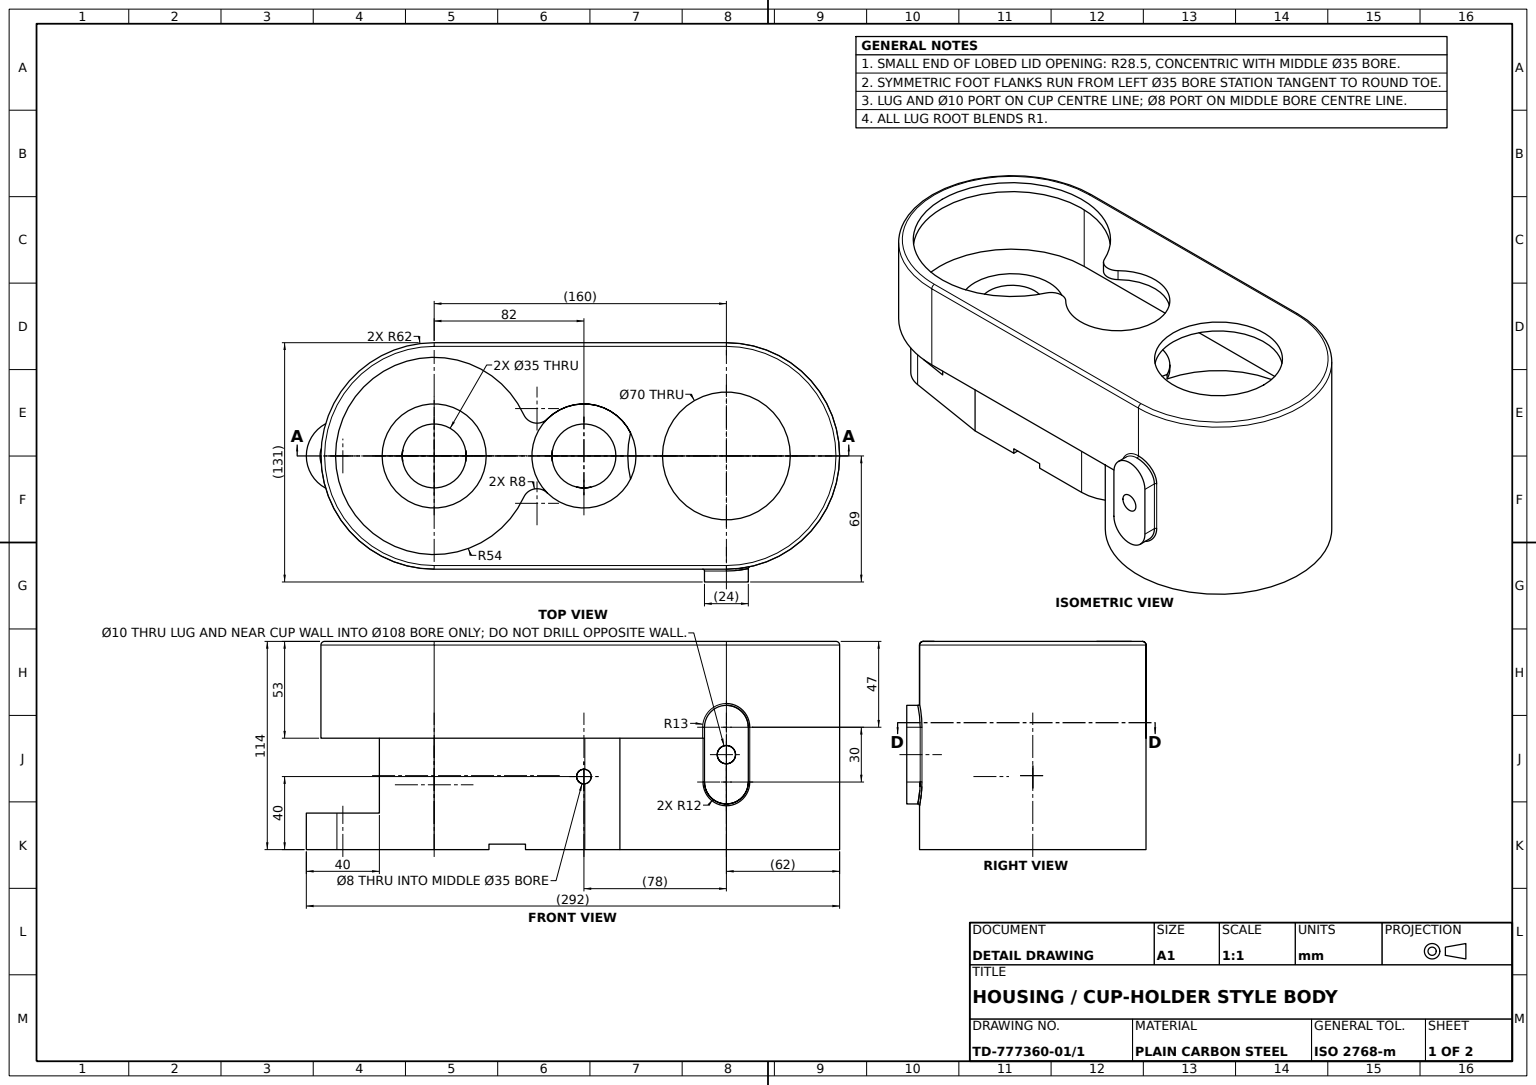
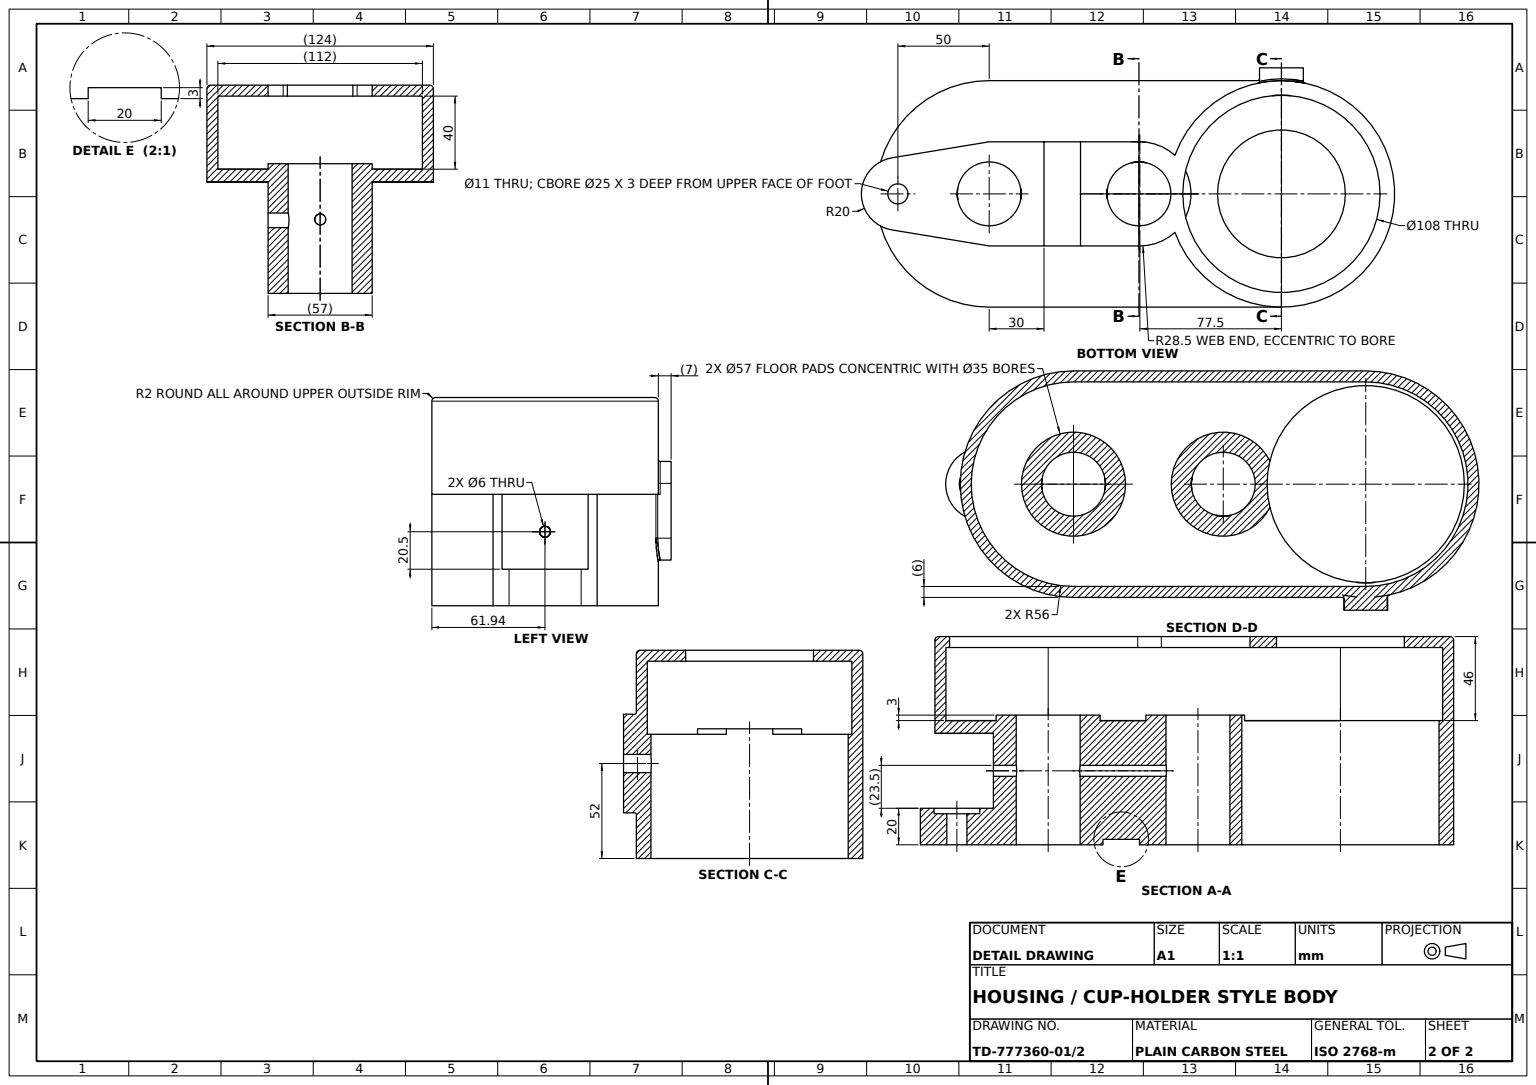
from build123d import *

# Parameters (mm, degrees)
HOUSING_OUTLINE_SKETCH_R        = 54
HOUSING_UPPER_BODY_DEPTH        = 53
LOWER_HOUSING_CIRCLE_SKETCH_R   = 62
LOWER_HOUSING_124_DEPTH         = 114
MOUNTING_FOOT_DEPTH             = 61
FOOT_PROFILE_CUT_SKETCH_W       = 57
FOOT_PROFILE_CUT_SKETCH_H       = 41
FOOT_PROFILE_CUT_DEPTH          = 70
GEAR_CAVITY_POCKET_DEPTH        = 46
SKETCH8_4_R                     = 35
GEAR_CAVITY_SECONDARY_CUT_DEPTH = 265.083320185
GEAR_BORE_SKETCH_R              = 54
GEAR_BORE_108_DEPTH             = 248.725654707
SIDE_CLEARANCE_CUT_DEPTH        = 40
SHAFT_OPENING_CUT_REACH         = 249.726
SHAFT_OPENING_SKETCH_R          = 17.5
PARTITION_START                 = 3
PARTITION_RIB_SKETCH_R          = 28.5
PARTITION_RIB_DEPTH             = 3
RIB_NOTCH_SKETCH_R              = 17.5
RIB_SHAFT_NOTCH_DEPTH           = 3
SIDE_LUG_BOSS_REACH             = 290.196
SIDE_LUG_HOLE_10_REACH          = 290.196
SIDE_LUG_HOLE_10_END_RADIUS     = 54
SIDE_LUG_HOLE_SKETCH_R          = 5
FOOT_C_BORE_HOLE_11_D           = 11
FOOT_C_BORE_HOLE_11_DEPTH       = 24
FOOT_C_BORE_HOLE_11_CBORE_D     = 25
FOOT_C_BORE_HOLE_11_CBORE_DEPTH = 3
FOOT_PIN_HOLE_6_REACH           = 287.063
FOOT_PIN_HOLE_6_END_RADIUS      = 17.5
FOOT_PIN_HOLE_SKETCH_R          = 3
SIDE_HOLE_8_REACH               = 267.814
SIDE_HOLE_SKETCH_R              = 4
SIDE_RELIEF_SLOT_DEPTH          = 266.813844705
SIDE_RELIEF_SLOT_DEPTH_BACK     = 266.813844705
SIDE_RELIEF_SLOT_SKETCH_W       = 20
SIDE_RELIEF_SLOT_SKETCH_H       = 3
SIDE_LUG_FILLET_R1_R            = 1
HOUSING_EDGE_FILLET_R2_R        = 2


with BuildPart() as part:
    # Housing Outline Sketch → Housing Upper Body (new body)
    with BuildSketch(Plane(origin=(0, 0, 0), x_dir=(1, 0, 0), z_dir=(0, 1, 0))):
        with BuildLine():
            Line((-62, 0), (-62, -160))
            ThreePointArc((-62, -160), (0, -222), (62, -160))
            Line((62, -160), (62, 0))
            ThreePointArc((62, 0), (0, 62), (-62, 0))
        make_face()
        with Locations(Location((0, 0, 0), (0, 0, 270))):
            Circle(HOUSING_OUTLINE_SKETCH_R, mode=Mode.SUBTRACT)
    extrude(amount=-HOUSING_UPPER_BODY_DEPTH)

    # Lower Housing Circle Sketch → Lower Housing _124 (add)
    with BuildSketch(Plane(origin=(0, 0, 0), x_dir=(1, 0, 0), z_dir=(0, 1, 0))):
        with Locations(Location((0, 0, 0), (0, 0, 270))):
            Circle(LOWER_HOUSING_CIRCLE_SKETCH_R)
    extrude(amount=-LOWER_HOUSING_124_DEPTH)

    # Mounting Foot Sketch → Mounting Foot (add)
    with BuildSketch(Plane.XZ.offset(53)):
        with BuildLine():
            Line((-28.5, 77.5), (-28.5, 160))
            Line((-28.5, 160), (-19.734400063, 213.248608036))
            ThreePointArc((-19.734400063, 213.248608036), (0, 230), (19.734400063, 213.248608036))
            Line((19.734400063, 213.248608036), (28.5, 160))
            Line((28.5, 160), (28.5, 77.5))
            ThreePointArc((28.5, 77.5), (0, 49), (-28.5, 77.5))
        make_face()
    extrude(amount=MOUNTING_FOOT_DEPTH)

    # Foot Profile Cut Sketch → Foot Profile Cut (cut)
    with BuildSketch(Plane.XY.offset(260)):
        with Locations((0, -73.5)):
            Rectangle(FOOT_PROFILE_CUT_SKETCH_W, FOOT_PROFILE_CUT_SKETCH_H)
    extrude(amount=-FOOT_PROFILE_CUT_DEPTH, mode=Mode.SUBTRACT)

    # Gear Cavity Sketch → Gear Cavity Pocket (cut)
    with BuildSketch(Plane(origin=(0, 0, 0), x_dir=(1, 0, 0), z_dir=(0, 1, 0))):
        with BuildLine():
            ThreePointArc((-22.587452566, -110.950973643), (-18.062041577, -105.111453337), (-20.249634035, -98.054982459))
            ThreePointArc((-20.249634035, -98.054982459), (0, -49.5), (20.249634035, -98.054982459))
            ThreePointArc((20.249634035, -98.054982459), (18.062041577, -105.111453337), (22.587452566, -110.950973643))
            ThreePointArc((22.587452566, -110.950973643), (0, -214), (-22.587452566, -110.950973643))
        make_face()
    extrude(amount=-GEAR_CAVITY_POCKET_DEPTH, mode=Mode.SUBTRACT)

    # Sketch8_4 → Gear Cavity Secondary Cut (cut, through all)
    with BuildSketch(Plane(origin=(0, 0, 0), x_dir=(1, 0, 0), z_dir=(0, 1, 0))):
        with Locations(Location((0, 0, 0), (0, 0, 270))):
            Circle(SKETCH8_4_R)
    extrude(amount=-GEAR_CAVITY_SECONDARY_CUT_DEPTH, mode=Mode.SUBTRACT)

    # Gear Bore Sketch → Gear Bore _108 (cut, through all)
    with BuildSketch(Plane(origin=(0, -46, 0), x_dir=(1, 0, 0), z_dir=(0, 1, 0))):
        with Locations(Location((0, 0, 0), (0, 0, 270))):
            Circle(GEAR_BORE_SKETCH_R)
    extrude(amount=-GEAR_BORE_108_DEPTH, mode=Mode.SUBTRACT)

    # Side Clearance Sketch → Side Clearance Cut (cut)
    with BuildSketch(Plane(origin=(0, -6, 0), x_dir=(1, 0, 0), z_dir=(0, 1, 0))):
        with BuildLine():
            Line((-56, 0), (-56, -160))
            ThreePointArc((-56, -160), (0, -216), (56, -160))
            Line((56, -160), (56, 0))
            ThreePointArc((56, 0), (0, 56), (-56, 0))
        make_face()
    extrude(amount=-SIDE_CLEARANCE_CUT_DEPTH, mode=Mode.SUBTRACT)

    # Shaft Opening Sketch → Shaft Opening Cut (cut, up to next)
    with BuildSketch(Plane(origin=(0, -46, 0), x_dir=(1, 0, 0), z_dir=(0, 1, 0)), mode=Mode.PRIVATE) as shaft_opening_cut_sk1:
        with Locations(Location((0, -78, 0), (0, 0, 270))):
            Circle(SHAFT_OPENING_SKETCH_R)
    shaft_opening_cut_tool1 = extrude(shaft_opening_cut_sk1.sketch, amount=-SHAFT_OPENING_CUT_REACH, mode=Mode.PRIVATE) & part.part
    # Shaft Opening Sketch → Shaft Opening Cut (cut, up to next)
    with BuildSketch(Plane(origin=(0, -46, 0), x_dir=(1, 0, 0), z_dir=(0, 1, 0)), mode=Mode.PRIVATE) as shaft_opening_cut_sk2:
        with Locations(Location((0, -160, 0), (0, 0, 270))):
            Circle(SHAFT_OPENING_SKETCH_R)
    shaft_opening_cut_tool2 = extrude(shaft_opening_cut_sk2.sketch, amount=-SHAFT_OPENING_CUT_REACH, mode=Mode.PRIVATE) & part.part
    add(shaft_opening_cut_tool1.solids().sort_by_distance((0, -46, 78))[0], mode=Mode.SUBTRACT)
    add(shaft_opening_cut_tool2.solids().sort_by_distance((0, -46, 160))[0], mode=Mode.SUBTRACT)

    # Partition Rib Sketch → Partition Rib (add)
    with BuildSketch(Plane(origin=(0, -46, 0), x_dir=(1, 0, 0), z_dir=(0, 1, 0)).offset(PARTITION_START)):
        with Locations(Location((0, -160, 0), (0, 0, 270))):
            Circle(PARTITION_RIB_SKETCH_R)
        with BuildLine():
            ThreePointArc((-12.698984804, -52.485576923), (0, -106.5), (12.698984804, -52.485576923))
            ThreePointArc((12.698984804, -52.485576923), (0, -54), (-12.698984804, -52.485576923))
        make_face()
    extrude(amount=-PARTITION_RIB_DEPTH)

    # Rib Notch Sketch → Rib Shaft Notch (cut)
    with BuildSketch(Plane(origin=(0, -43, 0), x_dir=(1, 0, 0), z_dir=(0, 1, 0))):
        with Locations(Location((0, -78, 0), (0, 0, 270))):
            Circle(RIB_NOTCH_SKETCH_R)
        with Locations(Location((0, -160, 0), (0, 0, 270))):
            Circle(RIB_NOTCH_SKETCH_R)
    extrude(amount=-RIB_SHAFT_NOTCH_DEPTH, mode=Mode.SUBTRACT)

    # Side Lug Sketch → Side Lug Boss (add, up to next)
    with BuildSketch(Plane(origin=(69, 0, 0), x_dir=(0, 0, -1), z_dir=(1, 0, 0)), mode=Mode.PRIVATE) as side_lug_boss_sk1:
        with BuildLine():
            Line((-12, -77), (-12, -47))
            ThreePointArc((-12, -47), (0, -35), (12, -47))
            Line((12, -47), (12, -77))
            ThreePointArc((12, -77), (0, -89), (-12, -77))
        make_face()
    side_lug_boss_tool1 = extrude(side_lug_boss_sk1.sketch, amount=-SIDE_LUG_BOSS_REACH, mode=Mode.PRIVATE) - part.part
    add(side_lug_boss_tool1.solids().sort_by_distance((69, -62, 0))[0])

    # Side Lug Hole _10: up to this cylinder (the profile starts outside it)
    side_lug_hole_10_end = Plane(origin=(0, -62, 0), z_dir=(0, 1, 0)) * Cylinder(SIDE_LUG_HOLE_10_END_RADIUS, 689.392, mode=Mode.PRIVATE)
    # Side Lug Hole Sketch → Side Lug Hole _10 (cut, up to the surface)
    with BuildSketch(Plane(origin=(69, 0, 0), x_dir=(0, 0, -1), z_dir=(1, 0, 0)), mode=Mode.PRIVATE) as side_lug_hole_10_sk1:
        with Locations((0, -62)):
            Circle(SIDE_LUG_HOLE_SKETCH_R)
    side_lug_hole_10_tool1 = extrude(side_lug_hole_10_sk1.sketch, amount=-SIDE_LUG_HOLE_10_REACH, mode=Mode.PRIVATE) - side_lug_hole_10_end
    add(side_lug_hole_10_tool1.solids().sort_by_distance((69, -62, 0))[0], mode=Mode.SUBTRACT)

    # Foot C-Bore Hole _11
    with Locations(Plane(origin=(0, -94, 0), x_dir=(1, 0, 0), z_dir=(0, 1, 0))):
        with Locations((0, -210)):
            CounterBoreHole(FOOT_C_BORE_HOLE_11_D / 2, FOOT_C_BORE_HOLE_11_CBORE_D / 2, FOOT_C_BORE_HOLE_11_CBORE_DEPTH, depth=FOOT_C_BORE_HOLE_11_DEPTH)

    # Foot Pin Hole _6: up to this cylinder (the profile starts outside it)
    foot_pin_hole_6_end = Plane(origin=(0, -73.5, 78), z_dir=(0, 1, 0)) * Cylinder(FOOT_PIN_HOLE_6_END_RADIUS, 610.126, mode=Mode.PRIVATE)
    # Foot Pin Hole Sketch → Foot Pin Hole _6 (cut, up to the surface)
    with BuildSketch(Plane.XY.offset(190), mode=Mode.PRIVATE) as foot_pin_hole_6_sk1:
        with Locations((-0.061504745, -73.5)):
            Circle(FOOT_PIN_HOLE_SKETCH_R)
    foot_pin_hole_6_tool1 = extrude(foot_pin_hole_6_sk1.sketch, amount=-FOOT_PIN_HOLE_6_REACH, mode=Mode.PRIVATE) - foot_pin_hole_6_end
    add(foot_pin_hole_6_tool1.solids().sort_by_distance((-0.061505, -73.5, 190))[0], mode=Mode.SUBTRACT)

    # Side Hole Sketch → Side Hole _8 (cut, up to next)
    with BuildSketch(Plane(origin=(0, 0, 0), x_dir=(0, 0, -1), z_dir=(1, 0, 0)), mode=Mode.PRIVATE) as side_hole_8_sk1:
        with Locations(Location((-78, -74, 0), (0, 0, 180))):
            Circle(SIDE_HOLE_SKETCH_R)
    side_hole_8_tool1 = extrude(side_hole_8_sk1.sketch, amount=SIDE_HOLE_8_REACH, mode=Mode.PRIVATE) & part.part
    add(side_hole_8_tool1.solids().sort_by_distance((0, -74, 78))[0], mode=Mode.SUBTRACT)

    # Side Relief Slot Sketch → Side Relief Slot (cut, two sides: drawn at the far end of the back side and taken through both)
    with BuildSketch(Plane(origin=(0, 0, 0), x_dir=(0, 0, -1), z_dir=(1, 0, 0)).offset(-SIDE_RELIEF_SLOT_DEPTH_BACK)):
        with Locations((-120, -112.5)):
            Rectangle(SIDE_RELIEF_SLOT_SKETCH_W, SIDE_RELIEF_SLOT_SKETCH_H)
    extrude(amount=SIDE_RELIEF_SLOT_DEPTH + SIDE_RELIEF_SLOT_DEPTH_BACK, mode=Mode.SUBTRACT)

    # Side Lug Fillet R1
    side_lug_fillet_r1_edges = [part.edges().sort_by_distance(p)[0] for p in [
        (61.416592464, -38.514846482, -8.48540924),
        (60.827625303, -62, -12),
        (62, -89, 0),
        (60.827625303, -65, 12),
        (62, -38.514718626, 8.485281374),
        (62, -50, 12),
    ]]
    fillet(side_lug_fillet_r1_edges, radius=SIDE_LUG_FILLET_R1_R)

    # Housing Edge Fillet R2
    housing_edge_fillet_r2_edges = [part.edges().sort_by_distance(p)[0] for p in [
        (0, 0, -62),
        (62, 0, 80),
        (0, 0, 222),
        (-62, 0, 80),
    ]]
    fillet(housing_edge_fillet_r2_edges, radius=HOUSING_EDGE_FILLET_R2_R)


solid = part.part
